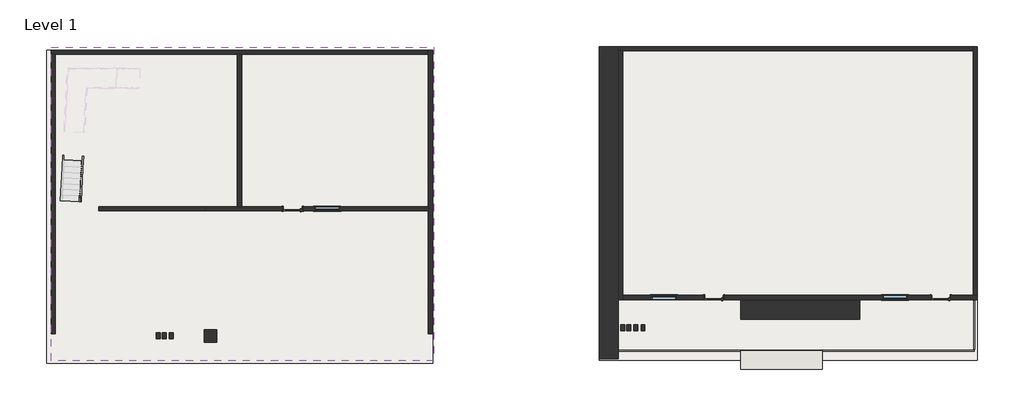
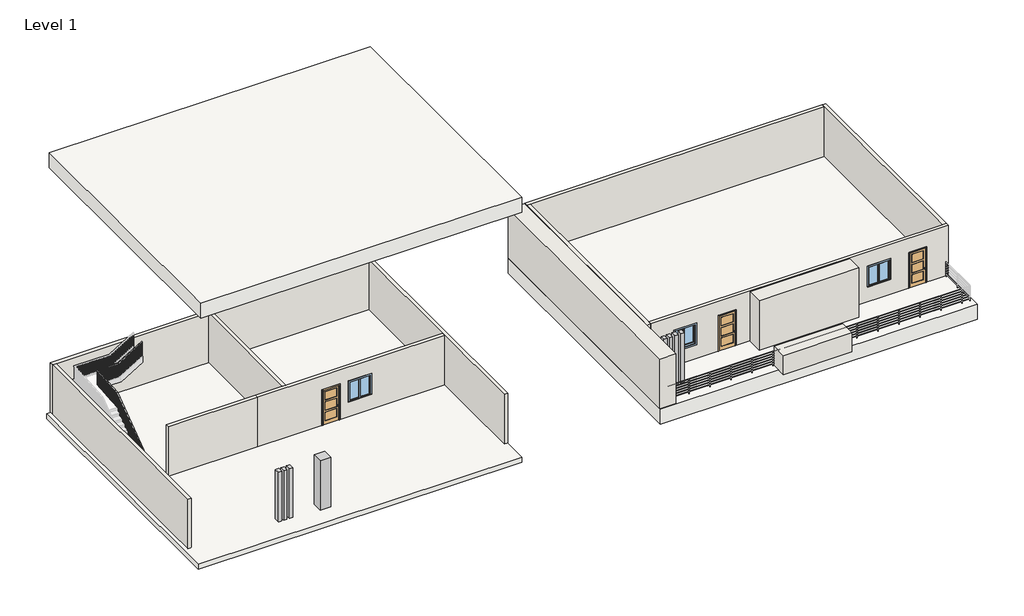
# One storey, part 1 of 3: 13 walls, 8 columns, 3 doors, 3 slabs, 3 windows, 1 railing.
"""IFC4 building model written with IfcOpenShell, lengths in millimetres."""

from ifc_helpers import new_model, si_unit, frame, origin, origin_with_axes, place, context, project, spatial, polyline, outline, extrude, faceted_brep, transform, mapped, element, save
from components import wood_timber_column_8_x_12_245a0583, door_54d869bf, window_3a1167bf, window_0862ab64

model = new_model("IFC4")

# Units and contexts
model_context = context("Model", 3, world=origin())
ifc_project = project(units=[si_unit("LENGTHUNIT", "METRE", prefix="MILLI")], contexts=[model_context])

# Site, building, storey
site = spatial("IfcSite", under=ifc_project)
building = spatial("IfcBuilding", under=site)
storey = spatial("IfcBuildingStorey", under=building, Name="Level 1", Elevation=0.0)

# Columns
placement = place(None, origin())
element("IfcColumn", 1, ObjectType="Rectangular Column : 24\" x 24\" 3", at=placement, inside=storey, context=model_context, shape_type="SweptSolid", body=[
    extrude(outline(polyline([(-12054.0621948, 4491.8216997), (-12054.0621948, 3882.2216997), (-12663.6621948, 3882.2216997), (-12663.6621948, 4491.8216997), (-12054.0621948, 4491.8216997)])), origin_with_axes(), (0.0, 0.0, 1.0), 3048.0),
])
wood_timber_column_8_x_12_shape = wood_timber_column_8_x_12_245a0583(model_context)
element("IfcColumn", 2, ObjectType="Wood Timber Column : 8 x 12", at=placement, inside=storey, context=model_context, shape_type="MappedRepresentation", body=[
    mapped(wood_timber_column_8_x_12_shape, transform((-14263.8621948, 4187.0216997, 0.0), x_axis=(1.0, 0.0, 0.0), y_axis=(0.0, 1.0, 0.0), z_axis=(0.0, 0.0, 1.0))),
])
element("IfcColumn", 3, ObjectType="Wood Timber Column : 8 x 12", at=placement, inside=storey, context=model_context, shape_type="MappedRepresentation", body=[
    mapped(wood_timber_column_8_x_12_shape, transform((-14594.0621948, 4187.0216997, 0.0), x_axis=(1.0, 0.0, 0.0), y_axis=(0.0, 1.0, 0.0), z_axis=(0.0, 0.0, 1.0))),
])
element("IfcColumn", 4, ObjectType="Wood Timber Column : 8 x 12", at=placement, inside=storey, context=model_context, shape_type="MappedRepresentation", body=[
    mapped(wood_timber_column_8_x_12_shape, transform((-14898.8621948, 4187.0216997, 0.0), x_axis=(1.0, 0.0, 0.0), y_axis=(0.0, 1.0, 0.0), z_axis=(0.0, 0.0, 1.0))),
])
element("IfcColumn", 5, ObjectType="Wood Timber Column : 8 x 12", at=placement, inside=storey, context=model_context, shape_type="MappedRepresentation", body=[
    mapped(wood_timber_column_8_x_12_shape, transform((8351.761019, 4590.8323495, 0.0), x_axis=(1.0, 0.0, 0.0), y_axis=(0.0, 1.0, 0.0), z_axis=(0.0, 0.0, 1.0))),
])
element("IfcColumn", 6, ObjectType="Wood Timber Column : 8 x 12", at=placement, inside=storey, context=model_context, shape_type="MappedRepresentation", body=[
    mapped(wood_timber_column_8_x_12_shape, transform((8021.561019, 4590.8323495, 0.0), x_axis=(1.0, 0.0, 0.0), y_axis=(0.0, 1.0, 0.0), z_axis=(0.0, 0.0, 1.0))),
])
element("IfcColumn", 7, ObjectType="Wood Timber Column : 8 x 12", at=placement, inside=storey, context=model_context, shape_type="MappedRepresentation", body=[
    mapped(wood_timber_column_8_x_12_shape, transform((7716.761019, 4590.8323495, 0.0), x_axis=(1.0, 0.0, 0.0), y_axis=(0.0, 1.0, 0.0), z_axis=(0.0, 0.0, 1.0))),
])
element("IfcColumn", 8, ObjectType="Wood Timber Column : 8 x 12", at=placement, inside=storey, context=model_context, shape_type="MappedRepresentation", body=[
    mapped(wood_timber_column_8_x_12_shape, transform((8707.361019, 4590.8323495, 0.0), x_axis=(1.0, 0.0, 0.0), y_axis=(0.0, 1.0, 0.0), z_axis=(0.0, 0.0, 1.0))),
])

# Doors
door_shape = door_54d869bf(model_context)
element("IfcDoor", 9, ObjectType="Door-Interior-Single-3_Panel_Vert-Wood : 36\" x 84\" 2", at=placement, inside=storey, context=model_context, shape_type="MappedRepresentation", body=[
    mapped(door_shape, transform((-8345.6621948, 10381.4466997, 0.0), x_axis=(-1.0, 0.0, 0.0), y_axis=(0.0, -1.0, 0.0), z_axis=(0.0, 0.0, 1.0))),
])
element("IfcDoor", 10, ObjectType="Door-Interior-Single-3_Panel_Vert-Wood : 36\" x 84\" 2", at=placement, inside=storey, context=model_context, shape_type="MappedRepresentation", body=[
    mapped(door_shape, transform((23217.111019, 6054.574368, 0.0), x_axis=(-1.0, 0.0, 0.0), y_axis=(0.0, -1.0, 0.0), z_axis=(0.0, 0.0, 1.0))),
])
element("IfcDoor", 11, ObjectType="Door-Interior-Single-3_Panel_Vert-Wood : 36\" x 84\" 2", at=placement, inside=storey, context=model_context, shape_type="MappedRepresentation", body=[
    mapped(door_shape, transform((12168.111019, 6054.574368, 0.0), x_axis=(-1.0, 0.0, 0.0), y_axis=(0.0, -1.0, 0.0), z_axis=(0.0, 0.0, 1.0))),
])

# Railing
element("IfcRailing", 12, ObjectType="Handrail - Rectangular", at=placement, inside=storey, context=model_context, shape_type="SolidModel", body=[
    faceted_brep([(-18751.6784827, 10722.0519913, 1083.7333333), (-18751.6784827, 10722.0519913, 1024.3318731), (-18700.9481023, 10719.3933247, 1024.3318731), (-18700.9481023, 10719.3933247, 1083.7333333), (-18576.2064886, 14070.2570954, 3115.7333333), (-18575.4637153, 14084.4300546, 3064.9333333), (-18524.7333349, 14081.7713881, 3064.9333333), (-18525.4761082, 14067.5984289, 3115.7333333), (-18458.2020473, 16321.9159704, 3115.7333333), (-18458.2020473, 16321.9159704, 3064.9333333), (-18409.9946473, 16271.1159704, 3064.9333333), (-18409.9946473, 16271.1159704, 3115.7333333), (-17229.733929, 16321.9159704, 3115.7333333), (-17215.5415195, 16321.9159704, 3064.9333333), (-17215.5415195, 16271.1159704, 3064.9333333), (-17229.733929, 16271.1159704, 3115.7333333), (-15832.733929, 16321.9159704, 3962.4), (-15832.733929, 16271.1159704, 3962.4), (-15832.733929, 16271.1159704, 3902.9985397), (-15832.733929, 16321.9159704, 3902.9985397)], [[[0, 1, 2, 3]], [[1, 0, 4, 5]], [[2, 1, 5, 6]], [[3, 2, 6, 7]], [[0, 3, 7, 4]], [[5, 4, 8, 9]], [[6, 5, 9, 10]], [[7, 6, 10, 11]], [[4, 7, 11, 8]], [[9, 8, 12, 13]], [[10, 9, 13, 14]], [[11, 10, 14, 15]], [[8, 11, 15, 12]], [[16, 17, 18, 19]], [[13, 12, 16, 19]], [[14, 13, 19, 18]], [[15, 14, 18, 17]], [[12, 15, 17, 16]]]),
    extrude(outline(polyline([(3862.5894488, -15899.408929), (3851.0439943, -15918.458929), (2878.6666667, -15918.458929), (2878.6666667, -15899.408929), (3862.5894488, -15899.408929)])), frame((0.0, 16286.9909704, 0.0), z_axis=(0.0, 1.0, 0.0), x_axis=(0.0, 0.0, 1.0)), (0.0, 0.0, 1.0), 19.05),
    extrude(outline(polyline([(3801.0136913, -16001.008929), (3789.4682367, -16020.058929), (2878.6666667, -16020.058929), (2878.6666667, -16001.008929), (3801.0136913, -16001.008929)])), frame((0.0, 16286.9909704, 0.0), z_axis=(0.0, 1.0, 0.0), x_axis=(0.0, 0.0, 1.0)), (0.0, 0.0, 1.0), 19.05),
    extrude(outline(polyline([(3739.4379337, -16102.608929), (3727.8924791, -16121.658929), (2878.6666667, -16121.658929), (2878.6666667, -16102.608929), (3739.4379337, -16102.608929)])), frame((0.0, 16286.9909704, 0.0), z_axis=(0.0, 1.0, 0.0), x_axis=(0.0, 0.0, 1.0)), (0.0, 0.0, 1.0), 19.05),
    extrude(outline(polyline([(3677.8621761, -16204.208929), (3666.3167216, -16223.258929), (2709.3333333, -16223.258929), (2709.3333333, -16204.208929), (3677.8621761, -16204.208929)])), frame((0.0, 16286.9909704, 0.0), z_axis=(0.0, 1.0, 0.0), x_axis=(0.0, 0.0, 1.0)), (0.0, 0.0, 1.0), 19.05),
    extrude(outline(polyline([(3616.2864185, -16305.808929), (3604.740964, -16324.858929), (2709.3333333, -16324.858929), (2709.3333333, -16305.808929), (3616.2864185, -16305.808929)])), frame((0.0, 16286.9909704, 0.0), z_axis=(0.0, 1.0, 0.0), x_axis=(0.0, 0.0, 1.0)), (0.0, 0.0, 1.0), 19.05),
    extrude(outline(polyline([(3554.710661, -16407.408929), (3543.1652064, -16426.458929), (2540.0, -16426.458929), (2540.0, -16407.408929), (3554.710661, -16407.408929)])), frame((0.0, 16286.9909704, 0.0), z_axis=(0.0, 1.0, 0.0), x_axis=(0.0, 0.0, 1.0)), (0.0, 0.0, 1.0), 19.05),
    extrude(outline(polyline([(3493.1349034, -16509.008929), (3481.5894488, -16528.058929), (2540.0, -16528.058929), (2540.0, -16509.008929), (3493.1349034, -16509.008929)])), frame((0.0, 16286.9909704, 0.0), z_axis=(0.0, 1.0, 0.0), x_axis=(0.0, 0.0, 1.0)), (0.0, 0.0, 1.0), 19.05),
    extrude(outline(polyline([(3431.5591458, -16610.608929), (3420.0136913, -16629.658929), (2540.0, -16629.658929), (2540.0, -16610.608929), (3431.5591458, -16610.608929)])), frame((0.0, 16286.9909704, 0.0), z_axis=(0.0, 1.0, 0.0), x_axis=(0.0, 0.0, 1.0)), (0.0, 0.0, 1.0), 19.05),
    extrude(outline(polyline([(3369.9833882, -16712.208929), (3358.4379337, -16731.258929), (2370.6666667, -16731.258929), (2370.6666667, -16712.208929), (3369.9833882, -16712.208929)])), frame((0.0, 16286.9909704, 0.0), z_axis=(0.0, 1.0, 0.0), x_axis=(0.0, 0.0, 1.0)), (0.0, 0.0, 1.0), 19.05),
    extrude(outline(polyline([(3308.4076307, -16813.808929), (3296.8621761, -16832.858929), (2370.6666667, -16832.858929), (2370.6666667, -16813.808929), (3308.4076307, -16813.808929)])), frame((0.0, 16286.9909704, 0.0), z_axis=(0.0, 1.0, 0.0), x_axis=(0.0, 0.0, 1.0)), (0.0, 0.0, 1.0), 19.05),
    extrude(outline(polyline([(3246.8318731, -16915.408929), (3235.2864185, -16934.458929), (2370.6666667, -16934.458929), (2370.6666667, -16915.408929), (3246.8318731, -16915.408929)])), frame((0.0, 16286.9909704, 0.0), z_axis=(0.0, 1.0, 0.0), x_axis=(0.0, 0.0, 1.0)), (0.0, 0.0, 1.0), 19.05),
    extrude(outline(polyline([(3185.2561155, -17017.008929), (3173.710661, -17036.058929), (2201.3333333, -17036.058929), (2201.3333333, -17017.008929), (3185.2561155, -17017.008929)])), frame((0.0, 16286.9909704, 0.0), z_axis=(0.0, 1.0, 0.0), x_axis=(0.0, 0.0, 1.0)), (0.0, 0.0, 1.0), 19.05),
    extrude(outline(polyline([(3123.6803579, -17118.608929), (3112.1349034, -17137.658929), (2201.3333333, -17137.658929), (2201.3333333, -17118.608929), (3123.6803579, -17118.608929)])), frame((0.0, 16286.9909704, 0.0), z_axis=(0.0, 1.0, 0.0), x_axis=(0.0, 0.0, 1.0)), (0.0, 0.0, 1.0), 19.05),
    extrude(outline(polyline([(-17326.0233473, 16286.9909704), (-17326.0233473, 16306.0409704), (-17306.9733473, 16306.0409704), (-17306.9733473, 16286.9909704), (-17326.0233473, 16286.9909704)])), frame((0.0, 0.0, 2201.3333333), z_axis=(0.0, 0.0, 1.0), x_axis=(1.0, 0.0, 0.0)), (0.0, 0.0, 1.0), 863.6),
    extrude(outline(polyline([(-17427.6233473, 16286.9909704), (-17427.6233473, 16306.0409704), (-17408.5733473, 16306.0409704), (-17408.5733473, 16286.9909704), (-17427.6233473, 16286.9909704)])), frame((0.0, 0.0, 2201.3333333), z_axis=(0.0, 0.0, 1.0), x_axis=(1.0, 0.0, 0.0)), (0.0, 0.0, 1.0), 863.6),
    extrude(outline(polyline([(-17529.2233473, 16286.9909704), (-17529.2233473, 16306.0409704), (-17510.1733473, 16306.0409704), (-17510.1733473, 16286.9909704), (-17529.2233473, 16286.9909704)])), frame((0.0, 0.0, 2201.3333333), z_axis=(0.0, 0.0, 1.0), x_axis=(1.0, 0.0, 0.0)), (0.0, 0.0, 1.0), 863.6),
    extrude(outline(polyline([(-17630.8233473, 16286.9909704), (-17630.8233473, 16306.0409704), (-17611.7733473, 16306.0409704), (-17611.7733473, 16286.9909704), (-17630.8233473, 16286.9909704)])), frame((0.0, 0.0, 2201.3333333), z_axis=(0.0, 0.0, 1.0), x_axis=(1.0, 0.0, 0.0)), (0.0, 0.0, 1.0), 863.6),
    extrude(outline(polyline([(-17732.4233473, 16286.9909704), (-17732.4233473, 16306.0409704), (-17713.3733473, 16306.0409704), (-17713.3733473, 16286.9909704), (-17732.4233473, 16286.9909704)])), frame((0.0, 0.0, 2201.3333333), z_axis=(0.0, 0.0, 1.0), x_axis=(1.0, 0.0, 0.0)), (0.0, 0.0, 1.0), 863.6),
    extrude(outline(polyline([(-17834.0233473, 16286.9909704), (-17834.0233473, 16306.0409704), (-17814.9733473, 16306.0409704), (-17814.9733473, 16286.9909704), (-17834.0233473, 16286.9909704)])), frame((0.0, 0.0, 2201.3333333), z_axis=(0.0, 0.0, 1.0), x_axis=(1.0, 0.0, 0.0)), (0.0, 0.0, 1.0), 863.6),
    extrude(outline(polyline([(-17935.6233473, 16286.9909704), (-17935.6233473, 16306.0409704), (-17916.5733473, 16306.0409704), (-17916.5733473, 16286.9909704), (-17935.6233473, 16286.9909704)])), frame((0.0, 0.0, 2201.3333333), z_axis=(0.0, 0.0, 1.0), x_axis=(1.0, 0.0, 0.0)), (0.0, 0.0, 1.0), 863.6),
    extrude(outline(polyline([(-18037.2233473, 16286.9909704), (-18037.2233473, 16306.0409704), (-18018.1733473, 16306.0409704), (-18018.1733473, 16286.9909704), (-18037.2233473, 16286.9909704)])), frame((0.0, 0.0, 2201.3333333), z_axis=(0.0, 0.0, 1.0), x_axis=(1.0, 0.0, 0.0)), (0.0, 0.0, 1.0), 863.6),
    extrude(outline(polyline([(-18138.8233473, 16286.9909704), (-18138.8233473, 16306.0409704), (-18119.7733473, 16306.0409704), (-18119.7733473, 16286.9909704), (-18138.8233473, 16286.9909704)])), frame((0.0, 0.0, 2201.3333333), z_axis=(0.0, 0.0, 1.0), x_axis=(1.0, 0.0, 0.0)), (0.0, 0.0, 1.0), 863.6),
    extrude(outline(polyline([(-18240.4233473, 16286.9909704), (-18240.4233473, 16306.0409704), (-18221.3733473, 16306.0409704), (-18221.3733473, 16286.9909704), (-18240.4233473, 16286.9909704)])), frame((0.0, 0.0, 2201.3333333), z_axis=(0.0, 0.0, 1.0), x_axis=(1.0, 0.0, 0.0)), (0.0, 0.0, 1.0), 863.6),
    extrude(outline(polyline([(-18342.0233473, 16286.9909704), (-18342.0233473, 16306.0409704), (-18322.9733473, 16306.0409704), (-18322.9733473, 16286.9909704), (-18342.0233473, 16286.9909704)])), frame((0.0, 0.0, 2201.3333333), z_axis=(0.0, 0.0, 1.0), x_axis=(1.0, 0.0, 0.0)), (0.0, 0.0, 1.0), 863.6),
    extrude(outline(polyline([(-18430.1638558, 16189.5932912), (-18449.1877485, 16190.5902912), (-18448.1907485, 16209.6141838), (-18429.1668559, 16208.6171838), (-18430.1638558, 16189.5932912)])), frame((0.0, 0.0, 2201.3333333), z_axis=(0.0, 0.0, 1.0), x_axis=(1.0, 0.0, 0.0)), (0.0, 0.0, 1.0), 863.6),
    extrude(outline(polyline([(-18435.481189, 16088.1325305), (-18454.5050816, 16089.1295304), (-18453.5080817, 16108.1534231), (-18434.484189, 16107.1564231), (-18435.481189, 16088.1325305)])), frame((0.0, 0.0, 2201.3333333), z_axis=(0.0, 0.0, 1.0), x_axis=(1.0, 0.0, 0.0)), (0.0, 0.0, 1.0), 863.6),
    extrude(outline(polyline([(-18440.7985222, 15986.6717697), (-18459.8224148, 15987.6687697), (-18458.8254148, 16006.6926623), (-18439.8015222, 16005.6956624), (-18440.7985222, 15986.6717697)])), frame((0.0, 0.0, 2201.3333333), z_axis=(0.0, 0.0, 1.0), x_axis=(1.0, 0.0, 0.0)), (0.0, 0.0, 1.0), 863.6),
    extrude(outline(polyline([(-18446.1158553, 15885.211009), (-18465.1397479, 15886.208009), (-18464.142748, 15905.2319016), (-18445.1188553, 15904.2349016), (-18446.1158553, 15885.211009)])), frame((0.0, 0.0, 2201.3333333), z_axis=(0.0, 0.0, 1.0), x_axis=(1.0, 0.0, 0.0)), (0.0, 0.0, 1.0), 863.6),
    extrude(outline(polyline([(-18451.4331885, 15783.7502483), (-18470.4570811, 15784.7472482), (-18469.4600811, 15803.7711409), (-18450.4361885, 15802.7741409), (-18451.4331885, 15783.7502483)])), frame((0.0, 0.0, 2201.3333333), z_axis=(0.0, 0.0, 1.0), x_axis=(1.0, 0.0, 0.0)), (0.0, 0.0, 1.0), 863.6),
    extrude(outline(polyline([(-18456.7505216, 15682.2894875), (-18475.7744143, 15683.2864875), (-18474.7774143, 15702.3103801), (-18455.7535216, 15701.3133802), (-18456.7505216, 15682.2894875)])), frame((0.0, 0.0, 2201.3333333), z_axis=(0.0, 0.0, 1.0), x_axis=(1.0, 0.0, 0.0)), (0.0, 0.0, 1.0), 863.6),
    extrude(outline(polyline([(-18462.0678548, 15580.8287268), (-18481.0917474, 15581.8257268), (-18480.0947474, 15600.8496194), (-18461.0708548, 15599.8526194), (-18462.0678548, 15580.8287268)])), frame((0.0, 0.0, 2201.3333333), z_axis=(0.0, 0.0, 1.0), x_axis=(1.0, 0.0, 0.0)), (0.0, 0.0, 1.0), 863.6),
    extrude(outline(polyline([(-18467.3851879, 15479.3679661), (-18486.4090806, 15480.364966), (-18485.4120806, 15499.3888587), (-18466.388188, 15498.3918587), (-18467.3851879, 15479.3679661)])), frame((0.0, 0.0, 2201.3333333), z_axis=(0.0, 0.0, 1.0), x_axis=(1.0, 0.0, 0.0)), (0.0, 0.0, 1.0), 863.6),
    extrude(outline(polyline([(-18472.7025211, 15377.9072053), (-18491.7264137, 15378.9042053), (-18490.7294137, 15397.9280979), (-18471.7055211, 15396.931098), (-18472.7025211, 15377.9072053)])), frame((0.0, 0.0, 2201.3333333), z_axis=(0.0, 0.0, 1.0), x_axis=(1.0, 0.0, 0.0)), (0.0, 0.0, 1.0), 863.6),
    extrude(outline(polyline([(-18478.0198542, 15276.4464446), (-18497.0437469, 15277.4434446), (-18496.0467469, 15296.4673372), (-18477.0228543, 15295.4703372), (-18478.0198542, 15276.4464446)])), frame((0.0, 0.0, 2201.3333333), z_axis=(0.0, 0.0, 1.0), x_axis=(1.0, 0.0, 0.0)), (0.0, 0.0, 1.0), 863.6),
    extrude(outline(polyline([(-18483.3371874, 15174.9856839), (-18502.36108, 15175.9826838), (-18501.3640801, 15195.0065765), (-18482.3401874, 15194.0095765), (-18483.3371874, 15174.9856839)])), frame((0.0, 0.0, 2201.3333333), z_axis=(0.0, 0.0, 1.0), x_axis=(1.0, 0.0, 0.0)), (0.0, 0.0, 1.0), 863.6),
    extrude(outline(polyline([(-18488.6545205, 15073.5249231), (-18507.6784132, 15074.5219231), (-18506.6814132, 15093.5458158), (-18487.6575206, 15092.5488158), (-18488.6545205, 15073.5249231)])), frame((0.0, 0.0, 2201.3333333), z_axis=(0.0, 0.0, 1.0), x_axis=(1.0, 0.0, 0.0)), (0.0, 0.0, 1.0), 863.6),
    extrude(outline(polyline([(-18493.9718537, 14972.0641624), (-18512.9957463, 14973.0611624), (-18511.9987464, 14992.085055), (-18492.9748537, 14991.0880551), (-18493.9718537, 14972.0641624)])), frame((0.0, 0.0, 2201.3333333), z_axis=(0.0, 0.0, 1.0), x_axis=(1.0, 0.0, 0.0)), (0.0, 0.0, 1.0), 863.6),
    extrude(outline(polyline([(-18499.2891868, 14870.6034017), (-18518.3130795, 14871.6004017), (-18517.3160795, 14890.6242943), (-18498.2921869, 14889.6272943), (-18499.2891868, 14870.6034017)])), frame((0.0, 0.0, 2201.3333333), z_axis=(0.0, 0.0, 1.0), x_axis=(1.0, 0.0, 0.0)), (0.0, 0.0, 1.0), 863.6),
    extrude(outline(polyline([(-18504.60652, 14769.142641), (-18523.6304126, 14770.1396409), (-18522.6334127, 14789.1635336), (-18503.60952, 14788.1665336), (-18504.60652, 14769.142641)])), frame((0.0, 0.0, 2201.3333333), z_axis=(0.0, 0.0, 1.0), x_axis=(1.0, 0.0, 0.0)), (0.0, 0.0, 1.0), 863.6),
    extrude(outline(polyline([(-18509.9238532, 14667.6818802), (-18528.9477458, 14668.6788802), (-18527.9507458, 14687.7027728), (-18508.9268532, 14686.7057729), (-18509.9238532, 14667.6818802)])), frame((0.0, 0.0, 2201.3333333), z_axis=(0.0, 0.0, 1.0), x_axis=(1.0, 0.0, 0.0)), (0.0, 0.0, 1.0), 863.6),
    extrude(outline(polyline([(-18515.2411863, 14566.2211195), (-18534.2650789, 14567.2181195), (-18533.268079, 14586.2420121), (-18514.2441863, 14585.2450121), (-18515.2411863, 14566.2211195)])), frame((0.0, 0.0, 2201.3333333), z_axis=(0.0, 0.0, 1.0), x_axis=(1.0, 0.0, 0.0)), (0.0, 0.0, 1.0), 863.6),
    extrude(outline(polyline([(-18520.5585195, 14464.7603588), (-18539.5824121, 14465.7573587), (-18538.5854121, 14484.7812514), (-18519.5615195, 14483.7842514), (-18520.5585195, 14464.7603588)])), frame((0.0, 0.0, 2201.3333333), z_axis=(0.0, 0.0, 1.0), x_axis=(1.0, 0.0, 0.0)), (0.0, 0.0, 1.0), 863.6),
    extrude(outline(polyline([(-18525.8758526, 14363.299598), (-18544.8997453, 14364.296598), (-18543.9027453, 14383.3204906), (-18524.8788527, 14382.3234907), (-18525.8758526, 14363.299598)])), frame((0.0, 0.0, 2201.3333333), z_axis=(0.0, 0.0, 1.0), x_axis=(1.0, 0.0, 0.0)), (0.0, 0.0, 1.0), 863.6),
    extrude(outline(polyline([(-18531.1931858, 14261.8388373), (-18550.2170784, 14262.8358373), (-18549.2200784, 14281.8597299), (-18530.1961858, 14280.8627299), (-18531.1931858, 14261.8388373)])), frame((0.0, 0.0, 2201.3333333), z_axis=(0.0, 0.0, 1.0), x_axis=(1.0, 0.0, 0.0)), (0.0, 0.0, 1.0), 863.6),
    extrude(outline(polyline([(-18536.5105189, 14160.3780766), (-18555.5344116, 14161.3750765), (-18554.5374116, 14180.3989692), (-18535.513519, 14179.4019692), (-18536.5105189, 14160.3780766)])), frame((0.0, 0.0, 2201.3333333), z_axis=(0.0, 0.0, 1.0), x_axis=(1.0, 0.0, 0.0)), (0.0, 0.0, 1.0), 863.6),
    extrude(outline(polyline([(222.8272727, -19.05), (234.3727273, 0.0), (1191.3561155, 0.0), (1191.3561155, -19.05), (222.8272727, -19.05)])), frame((-18547.1451852, 13957.4565551, 3223.3561155), z_axis=(-0.9986295347545738, 0.05233595624294526, 0.0), x_axis=(0.0, 0.0, -1.0)), (0.0, 0.0, 1.0), 19.05),
    extrude(outline(polyline([(222.8272727, -19.05), (234.3727272, 0.0), (1129.7803579, 0.0), (1129.7803579, -19.05), (222.8272727, -19.05)])), frame((-18552.4625184, 13855.9957944, 3161.7803579), z_axis=(-0.9986295347545738, 0.05233595624294526, 0.0), x_axis=(0.0, 0.0, -1.0)), (0.0, 0.0, 1.0), 19.05),
    extrude(outline(polyline([(222.8272728, -19.0500001), (234.3727273, 0.0), (1237.5379337, 0.0), (1237.5379337, -19.0500001), (222.8272728, -19.0500001)])), frame((-18557.7798515, 13754.5350336, 3100.2046004), z_axis=(-0.9986295347545738, 0.05233595624294526, 0.0), x_axis=(0.0, 0.0, -1.0)), (0.0, 0.0, 1.0), 19.05),
    extrude(outline(polyline([(222.8272728, -19.0500001), (234.3727273, 0.0), (1175.9621761, 0.0), (1175.9621761, -19.0500001), (222.8272728, -19.0500001)])), frame((-18563.0971847, 13653.0742729, 3038.6288428), z_axis=(-0.9986295347545738, 0.05233595624294526, 0.0), x_axis=(0.0, 0.0, -1.0)), (0.0, 0.0, 1.0), 19.05),
    extrude(outline(polyline([(222.8272727, -19.05), (234.3727273, 0.0), (1114.3864185, 0.0), (1114.3864185, -19.05), (222.8272727, -19.05)])), frame((-18568.4145179, 13551.6135122, 2977.0530852), z_axis=(-0.9986295347545738, 0.05233595624294526, 0.0), x_axis=(0.0, 0.0, -1.0)), (0.0, 0.0, 1.0), 19.05),
    extrude(outline(polyline([(222.8272727, -19.05), (234.3727272, 0.0), (1222.1439943, 0.0), (1222.1439943, -19.05), (222.8272727, -19.05)])), frame((-18573.731851, 13450.1527515, 2915.4773276), z_axis=(-0.9986295347545738, 0.05233595624294526, 0.0), x_axis=(0.0, 0.0, -1.0)), (0.0, 0.0, 1.0), 19.05),
    extrude(outline(polyline([(222.8272727, -19.0500001), (234.3727272, 0.0), (1160.5682367, 0.0), (1160.5682367, -19.0500001), (222.8272727, -19.0500001)])), frame((-18579.0491842, 13348.6919907, 2853.90157), z_axis=(-0.9986295347545738, 0.05233595624294526, 0.0), x_axis=(0.0, 0.0, -1.0)), (0.0, 0.0, 1.0), 19.05),
    extrude(outline(polyline([(222.8272728, -19.05), (234.3727273, 0.0), (1098.9924792, 0.0), (1098.9924792, -19.05), (222.8272728, -19.05)])), frame((-18584.3665173, 13247.23123, 2792.3258125), z_axis=(-0.9986295347545738, 0.05233595624294526, 0.0), x_axis=(0.0, 0.0, -1.0)), (0.0, 0.0, 1.0), 19.05),
    extrude(outline(polyline([(222.8272727, -19.05), (234.3727273, 0.0), (1206.7500549, 0.0), (1206.7500549, -19.05), (222.8272727, -19.05)])), frame((-18589.6838505, 13145.7704693, 2730.7500549), z_axis=(-0.9986295347545738, 0.05233595624294526, 0.0), x_axis=(0.0, 0.0, -1.0)), (0.0, 0.0, 1.0), 19.05),
    extrude(outline(polyline([(222.8272727, -19.0500001), (234.3727273, 0.0), (1145.1742973, 0.0), (1145.1742973, -19.0500001), (222.8272727, -19.0500001)])), frame((-18595.0011836, 13044.3097085, 2669.1742973), z_axis=(-0.9986295347545738, 0.05233595624294526, 0.0), x_axis=(0.0, 0.0, -1.0)), (0.0, 0.0, 1.0), 19.05),
    extrude(outline(polyline([(222.8272727, -19.05), (234.3727272, 0.0), (1083.5985397, 0.0), (1083.5985397, -19.05), (222.8272727, -19.05)])), frame((-18600.3185168, 12942.8489478, 2607.5985397), z_axis=(-0.9986295347545738, 0.05233595624294526, 0.0), x_axis=(0.0, 0.0, -1.0)), (0.0, 0.0, 1.0), 19.05),
    extrude(outline(polyline([(222.8272728, -19.05), (234.3727273, 0.0), (1191.3561155, 0.0), (1191.3561155, -19.05), (222.8272728, -19.05)])), frame((-18605.6358499, 12841.3881871, 2546.0227822), z_axis=(-0.9986295347545738, 0.05233595624294526, 0.0), x_axis=(0.0, 0.0, -1.0)), (0.0, 0.0, 1.0), 19.05),
    extrude(outline(polyline([(222.8272727, -19.0500001), (234.3727273, 0.0), (1129.7803579, 0.0), (1129.7803579, -19.0500001), (222.8272727, -19.0500001)])), frame((-18610.9531831, 12739.9274263, 2484.4470246), z_axis=(-0.9986295347545738, 0.05233595624294526, 0.0), x_axis=(0.0, 0.0, -1.0)), (0.0, 0.0, 1.0), 19.05),
    extrude(outline(polyline([(222.8272727, -19.05), (234.3727273, 0.0), (1237.5379337, 0.0), (1237.5379337, -19.05), (222.8272727, -19.05)])), frame((-18616.2705162, 12638.4666656, 2422.871267), z_axis=(-0.9986295347545738, 0.05233595624294526, 0.0), x_axis=(0.0, 0.0, -1.0)), (0.0, 0.0, 1.0), 19.05),
    extrude(outline(polyline([(222.8272727, -19.05), (234.3727272, 0.0), (1175.9621761, 0.0), (1175.9621761, -19.05), (222.8272727, -19.05)])), frame((-18621.5878494, 12537.0059049, 2361.2955094), z_axis=(-0.9986295347545738, 0.05233595624294526, 0.0), x_axis=(0.0, 0.0, -1.0)), (0.0, 0.0, 1.0), 19.05),
    extrude(outline(polyline([(222.8272728, -19.0500001), (234.3727273, 0.0), (1114.3864186, 0.0), (1114.3864186, -19.0500001), (222.8272728, -19.0500001)])), frame((-18626.9051826, 12435.5451441, 2299.7197519), z_axis=(-0.9986295347545738, 0.05233595624294526, 0.0), x_axis=(0.0, 0.0, -1.0)), (0.0, 0.0, 1.0), 19.05),
    extrude(outline(polyline([(222.8272727, -19.05), (234.3727273, 0.0), (1222.1439943, 0.0), (1222.1439943, -19.05), (222.8272727, -19.05)])), frame((-18632.2225157, 12334.0843834, 2238.1439943), z_axis=(-0.9986295347545738, 0.05233595624294526, 0.0), x_axis=(0.0, 0.0, -1.0)), (0.0, 0.0, 1.0), 19.05),
    extrude(outline(polyline([(222.8272727, -19.05), (234.3727273, 0.0), (1160.5682367, 0.0), (1160.5682367, -19.05), (222.8272727, -19.05)])), frame((-18637.5398489, 12232.6236227, 2176.5682367), z_axis=(-0.9986295347545738, 0.05233595624294526, 0.0), x_axis=(0.0, 0.0, -1.0)), (0.0, 0.0, 1.0), 19.05),
    extrude(outline(polyline([(222.8272727, -19.0500001), (234.3727272, 0.0), (1098.9924791, 0.0), (1098.9924791, -19.0500001), (222.8272727, -19.0500001)])), frame((-18642.857182, 12131.1628619, 2114.9924791), z_axis=(-0.9986295347545738, 0.05233595624294526, 0.0), x_axis=(0.0, 0.0, -1.0)), (0.0, 0.0, 1.0), 19.05),
    extrude(outline(polyline([(222.8272728, -19.0500001), (234.3727273, 0.0), (1206.7500549, 0.0), (1206.7500549, -19.0500001), (222.8272728, -19.0500001)])), frame((-18648.1745152, 12029.7021012, 2053.4167216), z_axis=(-0.9986295347545738, 0.05233595624294526, 0.0), x_axis=(0.0, 0.0, -1.0)), (0.0, 0.0, 1.0), 19.05),
    extrude(outline(polyline([(222.8272727, -19.05), (234.3727273, 0.0), (1145.1742973, 0.0), (1145.1742973, -19.05), (222.8272727, -19.05)])), frame((-18653.4918483, 11928.2413405, 1991.840964), z_axis=(-0.9986295347545738, 0.05233595624294526, 0.0), x_axis=(0.0, 0.0, -1.0)), (0.0, 0.0, 1.0), 19.05),
    extrude(outline(polyline([(222.8272727, -19.05), (234.3727273, 0.0), (1083.5985397, 0.0), (1083.5985397, -19.05), (222.8272727, -19.05)])), frame((-18658.8091815, 11826.7805798, 1930.2652064), z_axis=(-0.9986295347545738, 0.05233595624294526, 0.0), x_axis=(0.0, 0.0, -1.0)), (0.0, 0.0, 1.0), 19.05),
    extrude(outline(polyline([(222.8272727, -19.0500001), (234.3727272, 0.0), (1191.3561155, 0.0), (1191.3561155, -19.0500001), (222.8272727, -19.0500001)])), frame((-18664.1265146, 11725.319819, 1868.6894488), z_axis=(-0.9986295347545738, 0.05233595624294526, 0.0), x_axis=(0.0, 0.0, -1.0)), (0.0, 0.0, 1.0), 19.05),
    extrude(outline(polyline([(222.8272728, -19.05), (234.3727273, 0.0), (1129.780358, 0.0), (1129.780358, -19.05), (222.8272728, -19.05)])), frame((-18669.4438478, 11623.8590583, 1807.1136913), z_axis=(-0.9986295347545738, 0.05233595624294526, 0.0), x_axis=(0.0, 0.0, -1.0)), (0.0, 0.0, 1.0), 19.05),
    extrude(outline(polyline([(222.8272727, -19.05), (234.3727273, 0.0), (1237.5379337, 0.0), (1237.5379337, -19.05), (222.8272727, -19.05)])), frame((-18674.7611809, 11522.3982976, 1745.5379337), z_axis=(-0.9986295347545738, 0.05233595624294526, 0.0), x_axis=(0.0, 0.0, -1.0)), (0.0, 0.0, 1.0), 19.05),
    extrude(outline(polyline([(222.8272727, -19.0500001), (234.3727273, 0.0), (1175.9621761, 0.0), (1175.9621761, -19.0500001), (222.8272727, -19.0500001)])), frame((-18680.0785141, 11420.9375368, 1683.9621761), z_axis=(-0.9986295347545738, 0.05233595624294526, 0.0), x_axis=(0.0, 0.0, -1.0)), (0.0, 0.0, 1.0), 19.05),
    extrude(outline(polyline([(222.8272727, -19.05), (234.3727272, 0.0), (1114.3864185, 0.0), (1114.3864185, -19.05), (222.8272727, -19.05)])), frame((-18685.3958472, 11319.4767761, 1622.3864185), z_axis=(-0.9986295347545738, 0.05233595624294526, 0.0), x_axis=(0.0, 0.0, -1.0)), (0.0, 0.0, 1.0), 19.05),
    extrude(outline(polyline([(222.8272728, -19.05), (234.3727273, 0.0), (1222.1439943, 0.0), (1222.1439943, -19.05), (222.8272728, -19.05)])), frame((-18690.7131804, 11218.0160154, 1560.810661), z_axis=(-0.9986295347545738, 0.05233595624294526, 0.0), x_axis=(0.0, 0.0, -1.0)), (0.0, 0.0, 1.0), 19.05),
    extrude(outline(polyline([(222.8272727, -19.0500001), (234.3727273, 0.0), (1160.5682367, 0.0), (1160.5682367, -19.0500001), (222.8272727, -19.0500001)])), frame((-18696.0305136, 11116.5552546, 1499.2349034), z_axis=(-0.9986295347545738, 0.05233595624294526, 0.0), x_axis=(0.0, 0.0, -1.0)), (0.0, 0.0, 1.0), 19.05),
    extrude(outline(polyline([(222.8272727, -19.05), (234.3727273, 0.0), (1098.9924791, 0.0), (1098.9924791, -19.05), (222.8272727, -19.05)])), frame((-18701.3478467, 11015.0944939, 1437.6591458), z_axis=(-0.9986295347545738, 0.05233595624294526, 0.0), x_axis=(0.0, 0.0, -1.0)), (0.0, 0.0, 1.0), 19.05),
    extrude(outline(polyline([(222.8272727, -19.05), (234.3727272, 0.0), (1206.7500549, 0.0), (1206.7500549, -19.05), (222.8272727, -19.05)])), frame((-18706.6651799, 10913.6337332, 1376.0833882), z_axis=(-0.9986295347545738, 0.05233595624294526, 0.0), x_axis=(0.0, 0.0, -1.0)), (0.0, 0.0, 1.0), 19.05),
    extrude(outline(polyline([(222.8272728, -19.0500001), (234.3727273, 0.0), (1145.1742974, 0.0), (1145.1742974, -19.0500001), (222.8272728, -19.0500001)])), frame((-18711.982513, 10812.1729724, 1314.5076307), z_axis=(-0.9986295347545738, 0.05233595624294526, 0.0), x_axis=(0.0, 0.0, -1.0)), (0.0, 0.0, 1.0), 19.05),
    extrude(outline(polyline([(-17239.258929, 16286.9909704), (-17239.258929, 16306.0409704), (-17220.208929, 16306.0409704), (-17220.208929, 16286.9909704), (-17239.258929, 16286.9909704)])), frame((0.0, 0.0, 2201.3333333), z_axis=(0.0, 0.0, 1.0), x_axis=(1.0, 0.0, 0.0)), (0.0, 0.0, 1.0), 863.6),
    extrude(outline(polyline([(-18425.0849009, 16286.505524), (-18444.1087936, 16287.502524), (-18443.1117936, 16306.5264167), (-18424.087901, 16305.5294167), (-18425.0849009, 16286.505524)])), frame((0.0, 0.0, 2201.3333333), z_axis=(0.0, 0.0, 1.0), x_axis=(1.0, 0.0, 0.0)), (0.0, 0.0, 1.0), 863.6),
    extrude(outline(polyline([(-18541.8278521, 14058.9173158), (-18560.8517447, 14059.9143158), (-18559.8547448, 14078.9382084), (-18540.8308521, 14077.9412085), (-18541.8278521, 14058.9173158)])), frame((0.0, 0.0, 2201.3333333), z_axis=(0.0, 0.0, 1.0), x_axis=(1.0, 0.0, 0.0)), (0.0, 0.0, 1.0), 863.6),
    extrude(outline(polyline([(3902.9985397, -15832.733929), (3891.4530852, -15851.783929), (2878.6666667, -15851.783929), (2878.6666667, -15832.733929), (3902.9985397, -15832.733929)])), frame((0.0, 16286.9909704, 0.0), z_axis=(0.0, 1.0, 0.0), x_axis=(0.0, 0.0, 1.0)), (0.0, 0.0, 1.0), 19.05),
    extrude(outline(polyline([(222.8272728, -19.0500001), (234.3727273, 0.0), (1089.3712671, 0.0), (1089.3712671, -19.0500001), (222.8272728, -19.0500001)])), frame((-18716.8013462, 10720.224158, 1258.7046004), z_axis=(-0.9986295347545738, 0.05233595624294526, 0.0), x_axis=(0.0, 0.0, -1.0)), (0.0, 0.0, 1.0), 19.05),
])

# Slabs
element("IfcSlab", 13, ObjectType="Generic - 12\"", at=placement, inside=storey, context=model_context, shape_type="SweptSolid", body=[
    extrude(outline(polyline([(-1538.4621948, 18106.2216997), (-1538.4621948, 2855.2713631), (-20334.4621948, 2855.2713631), (-20334.4621948, 18106.2216997), (-1538.4621948, 18106.2216997)])), frame((0.0, 0.0, -304.8), z_axis=(0.0, 0.0, 1.0), x_axis=(1.0, 0.0, 0.0)), (0.0, 0.0, 1.0), 304.8),
])
element("IfcSlab", 14, ObjectType="Generic - 3'", at=placement, inside=storey, context=model_context, shape_type="SweptSolid", body=[
    extrude(outline(polyline([(24995.111019, 18275.149368), (24995.111019, 3009.749368), (6580.111019, 3009.749368), (6580.111019, 18275.149368), (24995.111019, 18275.149368)])), frame((0.0, 0.0, -914.4), z_axis=(0.0, 0.0, 1.0), x_axis=(1.0, 0.0, 0.0)), (0.0, 0.0, 1.0), 914.4),
])
element("IfcSlab", 15, ObjectType="Generic - 3'", at=placement, inside=storey, context=model_context, shape_type="SweptSolid", body=[
    extrude(outline(polyline([(-1471.688981, 18234.3145807), (-1471.688981, 2984.349368), (-20098.5750104, 2984.349368), (-20098.5750104, 18234.3145807), (-1471.688981, 18234.3145807)])), frame((0.0, 0.0, 14935.2), z_axis=(0.0, 0.0, 1.0), x_axis=(1.0, 0.0, 0.0)), (0.0, 0.0, 1.0), 914.4),
])

# Walls
element("IfcWall", 16, ObjectType="Generic - 3' 2", at=placement, inside=storey, context=model_context, shape_type="SweptSolid", body=[
    extrude(outline(polyline([(19254.711019, 4990.949368), (13463.511019, 4990.949368), (13463.511019, 5905.349368), (19254.711019, 5905.349368), (19254.711019, 4990.949368)])), origin_with_axes(), (0.0, 0.0, 1.0), 3048.0),
])
element("IfcWall", 17, ObjectType="Generic - 3' 4", at=placement, inside=storey, context=model_context, shape_type="SweptSolid", body=[
    extrude(outline(polyline([(17425.911019, 2552.549368), (13463.511019, 2552.549368), (13463.511019, 3466.949368), (17425.911019, 3466.949368), (17425.911019, 2552.549368)])), origin_with_axes(), (0.0, 0.0, 1.0), 1165.3811612),
])
element("IfcWall", 18, ObjectType="Generic - 3' 4", at=placement, inside=storey, context=model_context, shape_type="SweptSolid", body=[
    extrude(outline(polyline([(6580.111019, 3060.549368), (6580.111019, 18275.149368), (7494.511019, 18275.149368), (7494.511019, 3060.549368), (6580.111019, 3060.549368)])), origin_with_axes(), (0.0, 0.0, 1.0), 3048.0),
])
element("IfcWall", 19, ObjectType="Generic - 8\"", at=placement, inside=storey, context=model_context, shape_type="Brep", body=[
    faceted_brep([(-20105.8621948, 17903.0216997, 0.0), (-19902.6621948, 17903.0216997, 0.0), (-11038.0621948, 17903.0216997, 0.0), (-10834.8621948, 17903.0216997, 0.0), (-1741.6621948, 17903.0216997, 0.0), (-1741.6621948, 17903.0216997, 3048.0), (-10834.8621948, 17903.0216997, 3048.0), (-11038.0621948, 17903.0216997, 3048.0), (-19902.6621948, 17903.0216997, 3048.0), (-20105.8621948, 17903.0216997, 3048.0), (-20105.8621948, 18106.2216997, 0.0), (-20105.8621948, 18106.2216997, 3048.0), (-1741.6621948, 18106.2216997, 3048.0), (-1741.6621948, 18106.2216997, 0.0)], [[[0, 1, 2, 3, 4, 5, 6, 7, 8, 9]], [[10, 11, 12, 13]], [[4, 3, 2, 1, 0, 10, 13]], [[9, 8, 7, 6, 5, 12, 11]], [[0, 9, 11, 10]], [[5, 4, 13, 12]]]),
])
element("IfcWall", 20, ObjectType="Generic - 8\"", at=placement, inside=storey, context=model_context, shape_type="SweptSolid", body=[
    extrude(outline(polyline([(-19902.6621948, 17903.0216997), (-19902.6621948, 4288.6216997), (-20105.8621948, 4288.6216997), (-20105.8621948, 17903.0216997), (-19902.6621948, 17903.0216997)])), origin_with_axes(), (0.0, 0.0, 1.0), 3048.0),
])
element("IfcWall", 21, ObjectType="Generic - 8\"", at=placement, inside=storey, context=model_context, shape_type="Brep", body=[
    faceted_brep([(-1741.6621948, 18106.2216997, 0.0), (-1741.6621948, 17903.0216997, 0.0), (-1741.6621948, 10486.2216997, 0.0), (-1741.6621948, 10283.0216997, 0.0), (-1741.6621948, 4288.6216997, 0.0), (-1741.6621948, 4288.6216997, 3048.0), (-1741.6621948, 10283.0216997, 3048.0), (-1741.6621948, 10486.2216997, 3048.0), (-1741.6621948, 17903.0216997, 3048.0), (-1741.6621948, 18106.2216997, 3048.0), (-1538.4621948, 18106.2216997, 0.0), (-1538.4621948, 18106.2216997, 3048.0), (-1538.4621948, 4288.6216997, 3048.0), (-1538.4621948, 4288.6216997, 0.0)], [[[0, 1, 2, 3, 4, 5, 6, 7, 8, 9]], [[10, 11, 12, 13]], [[4, 3, 2, 1, 0, 10, 13]], [[5, 4, 13, 12]], [[9, 8, 7, 6, 5, 12, 11]], [[0, 9, 11, 10]]]),
])
element("IfcWall", 22, ObjectType="Generic - 8\"", at=placement, inside=storey, context=model_context, shape_type="SweptSolid", body=[
    extrude(outline(polyline([(-11038.0621948, 10486.2216997), (-11038.0621948, 17903.0216997), (-10834.8621948, 17903.0216997), (-10834.8621948, 10486.2216997), (-11038.0621948, 10486.2216997)])), origin_with_axes(), (0.0, 0.0, 1.0), 3048.0),
])
element("IfcWall", 23, ObjectType="Generic - 8\"", at=placement, inside=storey, context=model_context, shape_type="Brep", body=[
    faceted_brep([(-1741.6621948, 10283.0216997, 3048.0), (-12612.8621948, 10283.0216997, 3048.0), (-12612.8621948, 10283.0216997, 0.0), (-8828.2621948, 10283.0216997, 0.0), (-8828.2621948, 10283.0216997, 2159.0), (-7863.0621948, 10283.0216997, 2159.0), (-7863.0621948, 10283.0216997, 0.0), (-1741.6621948, 10283.0216997, 0.0), (-7278.8621948, 10283.0216997, 2133.6), (-6059.6621948, 10283.0216997, 2133.6), (-6059.6621948, 10283.0216997, 914.4), (-7278.8621948, 10283.0216997, 914.4), (-12612.8621948, 10486.2216997, 3048.0), (-11038.0621948, 10486.2216997, 3048.0), (-10834.8621948, 10486.2216997, 3048.0), (-1741.6621948, 10486.2216997, 3048.0), (-1741.6621948, 10486.2216997, 0.0), (-7863.0621948, 10486.2216997, 0.0), (-7863.0621948, 10486.2216997, 2159.0), (-8828.2621948, 10486.2216997, 2159.0), (-8828.2621948, 10486.2216997, 0.0), (-10834.8621948, 10486.2216997, 0.0), (-11038.0621948, 10486.2216997, 0.0), (-12612.8621948, 10486.2216997, 0.0), (-7278.8621948, 10486.2216997, 2133.6), (-7278.8621948, 10486.2216997, 914.4), (-6059.6621948, 10486.2216997, 914.4), (-6059.6621948, 10486.2216997, 2133.6)], [[[0, 1, 2, 3, 4, 5, 6, 7], [8, 9, 10, 11]], [[12, 13, 14, 15, 16, 17, 18, 19, 20, 21, 22, 23], [24, 25, 26, 27]], [[16, 7, 6, 17]], [[2, 23, 22, 21, 20, 3]], [[1, 0, 15, 14, 13, 12]], [[2, 1, 12, 23]], [[0, 7, 16, 15]], [[24, 27, 9, 8]], [[27, 26, 10, 9]], [[26, 25, 11, 10]], [[25, 24, 8, 11]], [[19, 4, 3, 20]], [[4, 19, 18, 5]], [[5, 18, 17, 6]]]),
])
element("IfcWall", 24, ObjectType="Generic - 8\"", at=placement, inside=storey, context=model_context, shape_type="Brep", body=[
    faceted_brep([(7519.911019, 18071.949368, 0.0), (7723.111019, 18071.949368, 0.0), (24791.911019, 18071.949368, 0.0), (24791.911019, 18071.949368, 3048.0), (7723.111019, 18071.949368, 3048.0), (7519.911019, 18071.949368, 3048.0), (7519.911019, 18275.149368, 0.0), (7519.911019, 18275.149368, 3048.0), (24791.911019, 18275.149368, 3048.0), (24791.911019, 18275.149368, 0.0)], [[[0, 1, 2, 3, 4, 5]], [[6, 7, 8, 9]], [[2, 1, 0, 6, 9]], [[5, 4, 3, 8, 7]], [[0, 5, 7, 6]], [[3, 2, 9, 8]]]),
])
element("IfcWall", 25, ObjectType="Generic - 8\"", at=placement, inside=storey, context=model_context, shape_type="Brep", body=[
    faceted_brep([(7723.111019, 6159.349368, 3048.0), (24791.911019, 6159.349368, 3048.0), (24995.111019, 6159.349368, 3048.0), (24995.111019, 6159.349368, 0.0), (24791.911019, 6159.349368, 0.0), (23699.711019, 6159.349368, 0.0), (23699.711019, 6159.349368, 2159.0), (22734.511019, 6159.349368, 2159.0), (22734.511019, 6159.349368, 0.0), (12650.711019, 6159.349368, 0.0), (12650.711019, 6159.349368, 2159.0), (11685.511019, 6159.349368, 2159.0), (11685.511019, 6159.349368, 0.0), (7723.111019, 6159.349368, 0.0), (9120.111019, 6159.349368, 2133.6), (9120.111019, 6159.349368, 914.4), (10339.311019, 6159.349368, 914.4), (10339.311019, 6159.349368, 2133.6), (20372.311019, 6159.349368, 2133.6), (20372.311019, 6159.349368, 914.4), (21591.511019, 6159.349368, 914.4), (21591.511019, 6159.349368, 2133.6), (24995.111019, 5956.149368, 3048.0), (7723.111019, 5956.149368, 3048.0), (7723.111019, 5956.149368, 0.0), (11685.511019, 5956.149368, 0.0), (11685.511019, 5956.149368, 2159.0), (12650.711019, 5956.149368, 2159.0), (12650.711019, 5956.149368, 0.0), (22734.511019, 5956.149368, 0.0), (22734.511019, 5956.149368, 2159.0), (23699.711019, 5956.149368, 2159.0), (23699.711019, 5956.149368, 0.0), (24995.111019, 5956.149368, 0.0), (9120.111019, 5956.149368, 2133.6), (10339.311019, 5956.149368, 2133.6), (10339.311019, 5956.149368, 914.4), (9120.111019, 5956.149368, 914.4), (20372.311019, 5956.149368, 2133.6), (21591.511019, 5956.149368, 2133.6), (21591.511019, 5956.149368, 914.4), (20372.311019, 5956.149368, 914.4)], [[[0, 1, 2, 3, 4, 5, 6, 7, 8, 9, 10, 11, 12, 13], [14, 15, 16, 17], [18, 19, 20, 21]], [[22, 23, 24, 25, 26, 27, 28, 29, 30, 31, 32, 33], [34, 35, 36, 37], [38, 39, 40, 41]], [[3, 33, 32, 5, 4]], [[8, 29, 28, 9]], [[24, 13, 12, 25]], [[2, 1, 0, 23, 22]], [[3, 2, 22, 33]], [[7, 30, 29, 8]], [[30, 7, 6, 31]], [[31, 6, 5, 32]], [[11, 26, 25, 12]], [[26, 11, 10, 27]], [[27, 10, 9, 28]], [[15, 14, 34, 37]], [[16, 15, 37, 36]], [[17, 16, 36, 35]], [[14, 17, 35, 34]], [[19, 18, 38, 41]], [[20, 19, 41, 40]], [[21, 20, 40, 39]], [[18, 21, 39, 38]], [[0, 13, 24, 23]]]),
])
element("IfcWall", 26, ObjectType="Generic - 8\"", at=placement, inside=storey, context=model_context, shape_type="Brep", body=[
    faceted_brep([(24791.911019, 18275.149368, 0.0), (24791.911019, 18071.949368, 0.0), (24791.911019, 6159.349368, 0.0), (24791.911019, 6159.349368, 3048.0), (24791.911019, 18071.949368, 3048.0), (24791.911019, 18275.149368, 3048.0), (24995.111019, 18275.149368, 0.0), (24995.111019, 18275.149368, 3048.0), (24995.111019, 6159.349368, 3048.0), (24995.111019, 6159.349368, 0.0)], [[[0, 1, 2, 3, 4, 5]], [[6, 7, 8, 9]], [[2, 1, 0, 6, 9]], [[5, 4, 3, 8, 7]], [[0, 5, 7, 6]], [[3, 2, 9, 8]]]),
])
element("IfcWall", 27, ObjectType="Generic - 8\"", at=placement, inside=storey, context=model_context, shape_type="Brep", body=[
    faceted_brep([(7723.111019, 5956.149368, 0.0), (7723.111019, 6159.349368, 0.0), (7723.111019, 18071.949368, 0.0), (7723.111019, 18071.949368, 3048.0), (7723.111019, 6159.349368, 3048.0), (7723.111019, 5956.149368, 3048.0), (7519.911019, 5956.149368, 0.0), (7519.911019, 5956.149368, 3048.0), (7519.911019, 18071.949368, 3048.0), (7519.911019, 18071.949368, 0.0)], [[[0, 1, 2, 3, 4, 5]], [[6, 7, 8, 9]], [[2, 1, 0, 6, 9]], [[5, 4, 3, 8, 7]], [[3, 2, 9, 8]], [[0, 5, 7, 6]]]),
])
element("IfcWall", 28, ObjectType="Generic - 8\" 2", at=placement, inside=storey, context=model_context, shape_type="SweptSolid", body=[
    extrude(outline(polyline([(-12612.8621948, 10283.0216997), (-17794.4621948, 10283.0216997), (-17794.4621948, 10486.2216997), (-12612.8621948, 10486.2216997), (-12612.8621948, 10283.0216997)])), origin_with_axes(), (0.0, 0.0, 1.0), 3048.0),
])

# Windows
window_shape = window_3a1167bf(model_context)
element("IfcWindow", 29, ObjectType="Casement Dbl with Trim : 48\" x 48\"", at=placement, inside=storey, context=model_context, shape_type="MappedRepresentation", body=[
    mapped(window_shape, transform((9729.711019, 6038.699368, 0.0), x_axis=(-1.0, 0.0, 0.0), y_axis=(0.0, -1.0, 0.0), z_axis=(0.0, 0.0, 1.0))),
])
window_2_shape = window_0862ab64(model_context)
element("IfcWindow", 30, ObjectType="Casement Dbl with Trim : 48\" x 48\" 2", at=placement, inside=storey, context=model_context, shape_type="MappedRepresentation", body=[
    mapped(window_2_shape, transform((-6669.2621948, 10403.6716997, 0.0), x_axis=(-1.0, 0.0, 0.0), y_axis=(0.0, -1.0, 0.0), z_axis=(0.0, 0.0, 1.0))),
])
element("IfcWindow", 31, ObjectType="Casement Dbl with Trim : 48\" x 48\" 2", at=placement, inside=storey, context=model_context, shape_type="MappedRepresentation", body=[
    mapped(window_2_shape, transform((20981.911019, 6076.799368, 0.0), x_axis=(-1.0, 0.0, 0.0), y_axis=(0.0, -1.0, 0.0), z_axis=(0.0, 0.0, 1.0))),
])

save(model, "model.ifc")

# Revit data of these elements
# Type "Rectangular Column : 24\" x 24\" 3"
#   Assembly Code = "B1010200"
#   Depth = 2' - 0"
#   Offset Base = 0' - 0"
#   Offset Top = 0' - 0"
#   Width = 2' - 0"
#   built-in parameter 1002110 = 12443391
#   Material = Paint - Sienna
# Type "Wood Timber Column : 8 x 12"
#   Assembly Code = "B1010200"
#   Depth = 0' - 11 1/2"
#   Width = 0' - 7 1/2"
#   Material = Softwood, Lumber
# Type "Door-Interior-Single-3_Panel_Vert-Wood : 36\" x 84\" 2"
#   Type Mark = "11"
#   Assembly Code = "C1020300"
#   Analytic Construction = "Wooden"
#   Top Rail = 0' - 4 11/16"
#   Thickness = 0' - 1 3/8"
#   Thermal Resistance (R) = 2.5876 (h·ft²·°F)/BTU
#   Swing Angle [instance default] = 90.00°
#   Stiles = 0' - 4 3/4"
#   Rough Width = 3' - 2"
#   Rough Height = 7' - 1"
#   Intermediate Rail = 0' - 4 1/2"
#   Height = 7' - 0"
#   Width = 3' - 0"
#   Heat Transfer Coefficient (U) = 0.3865 BTU/(h·ft²·°F)
#   Bottom Rail = 0' - 9 1/8"
#   Trim Material = Cherry
#   Panel Material = Door - Panel
#   Frame Material = Door - Panel
#   Door Handle Material = Aluminum
#   Visual Light Transmittance = 0
#   Solar Heat Gain Coefficient = 0
#   Wall Closure = (empty or 0)
#   Function = (empty or 0)
# Type "Handrail - Rectangular"
#   Assembly Code = "C2010400"
#   built-in parameter 1008612 = 0.0416667 (stored number, unit not read)
#   built-in parameter 1008611 = 0.0416667 (stored number, unit not read)
#   built-in parameter 1008609 = 0.333333 (stored number, unit not read)
#   built-in parameter 1008604 = 0.166667 (stored number, unit not read)
#   built-in parameter 1008603 = 0.166667 (stored number, unit not read)
#   Railing Height = 3' - 0"
#   built-in parameter 1008630 = 2
#   built-in parameter 1008610 = 2
#   built-in parameter 1008618 = Baluster - Square : 3/4"
# Type "Generic - 12\""
#   Assembly Code = "B1010"
#   Function = 0
#   Layers, outside or top first: 1' - 0" no material (function 1)
# Type "Generic - 3'"
#   Assembly Code = "B1010"
#   Function = 0
#   Layers, outside or top first: 3' - 0" "Parking Stripe" (function 1)
# Type "Generic - 3' 2"
#   Assembly Code = "B2010"
#   Layers, outside or top first: 3' - 0" "Asphalt Shingle" (function 1)
# Type "Generic - 3' 4"
#   Assembly Code = "B2010"
#   Layers, outside or top first: 3' - 0" "Parking Stripe" (function 1)
# Type "Generic - 8\""
#   Assembly Code = "B2010"
#   Layers, outside or top first: 0' - 8" "Paint - Sienna" (function 1)
# Type "Generic - 8\" 2"
#   Assembly Code = "B2010"
#   Layers, outside or top first: 0' - 8" "Brick, Common" (function 1)
# Type "Casement Dbl with Trim : 48\" x 48\""
#   Type Mark = "10"
#   Construction Type Id = "GSP4R"
#   Assembly Code = "B2020100"
#   Analytic Construction = "1/8 in Pilkington single glazing"
#   Visual Light Transmittance = 0.9
#   Thermal Resistance (R) = 1.53941 (h·ft²·°F)/BTU
#   Solar Heat Gain Coefficient = 0.78
#   Heat Transfer Coefficient (U) = 0.6496 BTU/(h·ft²·°F)
#   Height = 4' - 0"
#   Default Sill Height = 3' - 0"
#   Trim Projection - Ext. = 0' - 0 1/2"
#   Trim Projection - Int. = 0' - 0 3/4"
#   Trim Width - Exterior = 0' - 3 1/2"
#   Trim Width - Interior = 0' - 3 1/2"
#   Width = 4' - 0"
#   Window Inset = 0' - 0 3/4"
#   Define Thermal Properties by = 1
#   Glass Pane Material = Glass
#   Sash Material = Sash
#   Trim Exterior Material = Trim
#   Trim Interior Material = Trim
#   Wall Closure = (empty or 0)
# Type "Casement Dbl with Trim : 48\" x 48\" 2"
#   Type Mark = "13"
#   Construction Type Id = "GSP4R"
#   Assembly Code = "B2020100"
#   Analytic Construction = "1/8 in Pilkington single glazing"
#   Visual Light Transmittance = 0.9
#   Thermal Resistance (R) = 1.53941 (h·ft²·°F)/BTU
#   Solar Heat Gain Coefficient = 0.78
#   Heat Transfer Coefficient (U) = 0.6496 BTU/(h·ft²·°F)
#   Height = 4' - 0"
#   Default Sill Height = 3' - 0"
#   Trim Projection - Ext. = 0' - 0 1/2"
#   Trim Projection - Int. = 0' - 0 3/4"
#   Trim Width - Exterior = 0' - 3 1/2"
#   Trim Width - Interior = 0' - 3 1/2"
#   Width = 4' - 0"
#   Window Inset = 0' - 0 3/4"
#   Define Thermal Properties by = 1
#   Glass Pane Material = Glass, Clear Glazing
#   Sash Material = Copper
#   Trim Exterior Material = Earth
#   Trim Interior Material = Earth
#   Wall Closure = (empty or 0)
# Element 1 (IfcColumn, "Rectangular Column : 24\" x 24\" 3")
#   Phase Created = New Construction
#   Materials on its faces: "Paint - Sienna"
# Elements 2, 3, 4, 5, 6, 7, 8 (IfcColumn, "Wood Timber Column : 8 x 12")
#   Phase Created = New Construction
#   Materials on its faces: "Softwood, Lumber"
# Elements 9, 10, 11 (IfcDoor, "Door-Interior-Single-3_Panel_Vert-Wood : 36\" x 84\" 2")
#   Swing Angle = 90.00°
#   Phase Created = New Construction
#   Materials on its faces: "Door - Panel", "Aluminum", "Cherry"
# Element 12 (IfcRailing, "Handrail - Rectangular")
#   Phase Created = New Construction
# Element 13 (IfcSlab, "Generic - 12\"")
#   Height Offset From Level = 0' - 0"
#   Phase Created = New Construction
#   Materials on its faces: "Default Floor"
# Element 14 (IfcSlab, "Generic - 3'")
#   Height Offset From Level = 0' - 0"
#   Phase Created = New Construction
#   Materials on its faces: "Parking Stripe"
# Element 15 (IfcSlab, "Generic - 3'")
#   Height Offset From Level = 52' - 0"
#   Phase Created = New Construction
#   Materials on its faces: "Parking Stripe"
# Element 16 (IfcWall, "Generic - 3' 2")
#   Top Offset = 0' - 0"
#   Base Offset = 0' - 0"
#   Unconnected Height = 10' - 0"
#   wall height = 10' - 0"
#   Phase Created = New Construction
#   Base Constraint = Level 1
#   Materials on its faces: "Asphalt Shingle"
# Element 17 (IfcWall, "Generic - 3' 4")
#   Top Offset = 0' - 0"
#   Base Offset = 0' - 0"
#   Unconnected Height = 3' - 9.88115"
#   wall height = 3' - 9.88115"
#   Phase Created = New Construction
#   Base Constraint = Level 1
#   Materials on its faces: "Parking Stripe"
# Element 18 (IfcWall, "Generic - 3' 4")
#   Top Offset = 0' - 0"
#   Base Offset = 0' - 0"
#   Unconnected Height = 10' - 0"
#   wall height = 10' - 0"
#   Phase Created = New Construction
#   Base Constraint = Level 1
#   Materials on its faces: "Parking Stripe"
# Elements 19, 20, 21, 22, 23, 24, 25, 26, 27 (IfcWall, "Generic - 8\"")
#   Top Offset = 0' - 0"
#   Base Offset = 0' - 0"
#   Unconnected Height = 10' - 0"
#   wall height = 10' - 0"
#   Phase Created = New Construction
#   Base Constraint = Level 1
#   Materials on its faces: "Paint - Sienna"
# Element 28 (IfcWall, "Generic - 8\" 2")
#   Top Offset = 0' - 0"
#   Base Offset = 0' - 0"
#   Unconnected Height = 10' - 0"
#   wall height = 10' - 0"
#   Phase Created = New Construction
#   Base Constraint = Level 1
#   Materials on its faces: "Brick, Common"
# Element 29 (IfcWindow, "Casement Dbl with Trim : 48\" x 48\"")
#   Mark = "2"
#   Phase Created = New Construction
#   Materials on its faces: "Sash", "Trim", "Glass"
# Element 30 (IfcWindow, "Casement Dbl with Trim : 48\" x 48\" 2")
#   Mark = "1"
#   Phase Created = New Construction
#   Materials on its faces: "Copper", "Earth", "Glass, Clear Glazing"
# Element 31 (IfcWindow, "Casement Dbl with Trim : 48\" x 48\" 2")
#   Mark = "3"
#   Phase Created = New Construction
#   Materials on its faces: "Copper", "Earth", "Glass, Clear Glazing"
# Materials
#   "Paint - Sienna": colour RGB 255 255 255, transparency 0, Cost = 0
#   "Softwood, Lumber": class "Wood", colour RGB 223 192 134, transparency 0, Description = "Pinus Echinata", Cost = 0
#   "Cherry": class "Wood", colour RGB 226 177 128, transparency 0, Description = "Prunus Serotina", Cost = 0
#   "Door - Panel": class "Wood", colour RGB 210 159 95, transparency 0
#   "Aluminum": class "Metal", colour RGB 247 247 247, transparency 0, Description = "Aluminum 6061", Cost = 0
#   "Parking Stripe": class "Paint", colour RGB 255 221 187, transparency 0, Cost = 0
#   "Asphalt Shingle": class "Generic", colour RGB 155 155 155, transparency 0, Description = "Asphalt roofing shingle", Cost = 0
#   "Brick, Common": class "Masonry", colour RGB 170 98 104, transparency 0, Description = "Common brick", Cost = 0
#   "Glass": class "Glass", colour RGB 0 128 192, transparency 0.75, Description = "Soda Lime Glass", Cost = 0
#   "Sash": class "Wood", colour RGB 224 178 126, transparency 0
#   "Trim": class "Wood", colour RGB 224 178 126, transparency 0
#   "Glass, Clear Glazing": class "Glass", colour RGB 0 128 192, transparency 0.75, Description = "Clear glazing", Cost = 0
#   "Copper": class "Metal", colour RGB 0 0 0, transparency 0, Description = "Copper, matte finish", Cost = 0
#   "Earth": class "Generic", colour RGB 97 75 62, transparency 0, Description = "Soil", Cost = 0
#   "Default Floor": colour RGB 128 128 128, transparency 0
